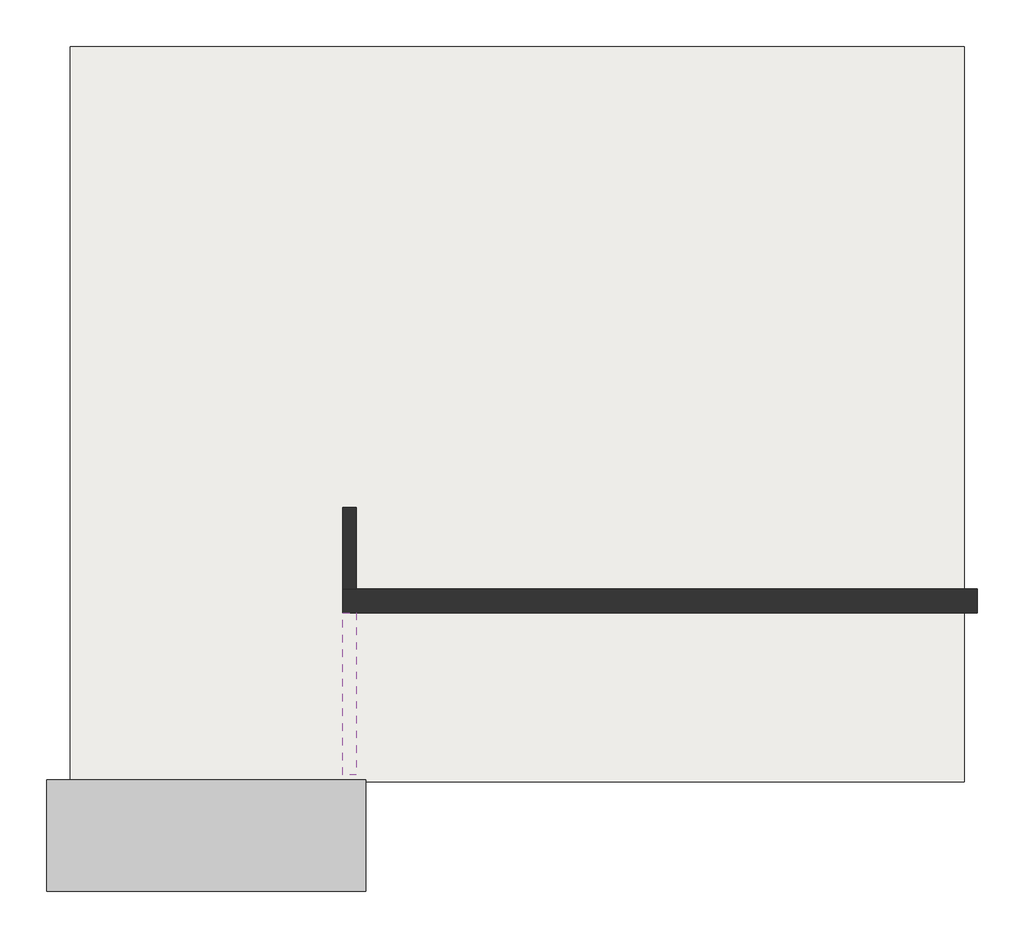
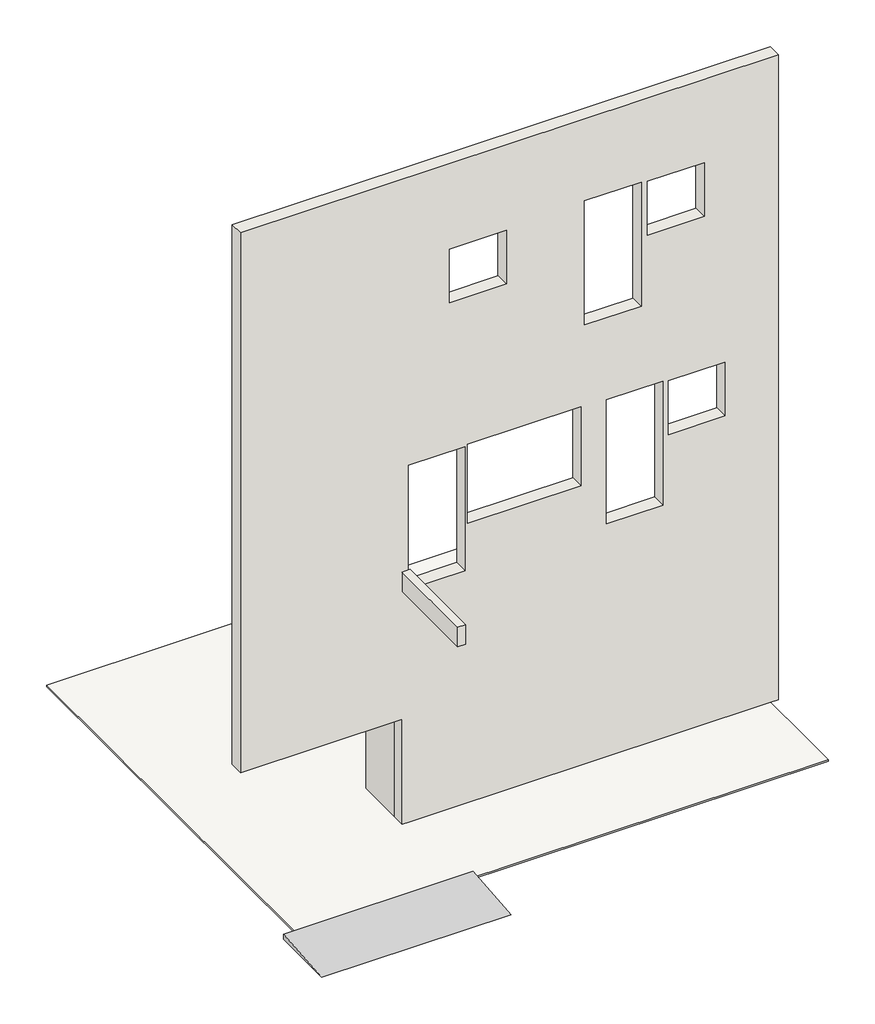
# One storey: 3 walls, 1 ramp, 1 slab.
"""IFC4 building model written with IfcOpenShell, lengths in millimetres."""

from ifc_helpers import new_model, si_unit, frame, origin, place, context, project, spatial, polyline, outline, extrude, faceted_brep, transform, mapped, element, save
from components import standard_ef43e6ca

model = new_model("IFC4")

# Units and contexts
model_context = context("Model", 3, world=origin())
ifc_project = project(units=[si_unit("LENGTHUNIT", "METRE", prefix="MILLI")], contexts=[model_context])

# Site, building, storey
site = spatial("IfcSite", under=ifc_project)
building = spatial("IfcBuilding", under=site)
storey = spatial("IfcBuildingStorey", under=building, Elevation=914.4)

# Ramp
placement = place(None, origin())
standard_shape = standard_ef43e6ca(model_context)
element("IfcRamp", 1, ObjectType="Standard", at=placement, inside=storey, context=model_context, shape_type="MappedRepresentation", body=[
    mapped(standard_shape, transform((0.0, 0.0, 0.0), x_axis=(1.0, 0.0, 0.0), y_axis=(0.0, 1.0, 0.0), z_axis=(0.0, 0.0, 1.0))),
])

# Slab
element("IfcSlab", 2, ObjectType="2\"", at=placement, inside=storey, context=model_context, shape_type="SweptSolid", body=[
    extrude(outline(polyline([(9321.1305046, -1515.8053244), (9321.1305046, -8538.9053244), (788.1495839, -8538.9053244), (788.1495839, -1515.8053244), (9321.1305046, -1515.8053244)])), frame((0.0, 0.0, 889.0), z_axis=(0.0, 0.0, 1.0), x_axis=(1.0, 0.0, 0.0)), (0.0, 0.0, 1.0), 25.4),
])

# Walls
element("IfcWall", 3, ObjectType="5\"", at=placement, inside=storey, context=model_context, shape_type="SweptSolid", body=[
    extrude(outline(polyline([(3517.0722446, -6926.0053244), (3517.0722446, -8475.4053244), (3390.0722446, -8475.4053244), (3390.0722446, -6926.0053244), (3517.0722446, -6926.0053244)])), frame((0.0, 0.0, 4876.8), z_axis=(0.0, 0.0, 1.0), x_axis=(1.0, 0.0, 0.0)), (0.0, 0.0, 1.0), 330.2),
])
element("IfcWall", 4, ObjectType="5\"", at=placement, inside=storey, context=model_context, shape_type="Brep", body=[
    faceted_brep([(3517.0722446, -6697.4053244, 4648.2), (3517.0722446, -6697.4053244, 914.4), (3517.0722446, -5918.2703867, 914.4), (3517.0722446, -5918.2703867, 4648.2), (3390.0722446, -6697.4053244, 914.4), (3390.0722446, -6697.4053244, 2706.0311436), (3390.0722446, -6697.4053244, 4648.2), (3390.0722446, -5918.2703867, 4648.2), (3390.0722446, -5918.2703867, 914.4)], [[[0, 1, 2, 3]], [[4, 5, 6, 7, 8]], [[2, 1, 4, 8]], [[3, 2, 8, 7]], [[0, 3, 7, 6]], [[0, 6, 5, 4, 1]]]),
])
element("IfcWall", 5, ObjectType="9\"", at=placement, inside=storey, context=model_context, shape_type="Brep", body=[
    faceted_brep([(3390.0722446, -6926.0053244, 914.4), (3517.0722446, -6926.0053244, 914.4), (9321.1305046, -6926.0053244, 914.4), (9448.1305046, -6926.0053244, 914.4), (9448.1305046, -6926.0053244, 4648.2), (9448.1305046, -6926.0053244, 11658.6), (9448.1305046, -6926.0053244, 11887.2), (788.1495839, -6926.0053244, 11887.2), (788.1495839, -6926.0053244, 11658.6), (788.1495839, -6926.0053244, 2706.0311436), (3390.0722446, -6926.0053244, 2706.0311436), (6328.3305046, -6926.0053244, 8382.0), (6328.3305046, -6926.0053244, 10492.0), (7238.3305046, -6926.0053244, 10492.0), (7238.3305046, -6926.0053244, 8382.0), (7339.9305046, -6926.0053244, 9555.3436332), (7339.9305046, -6926.0053244, 10469.7436332), (8254.3305046, -6926.0053244, 10469.7436332), (8254.3305046, -6926.0053244, 9555.3436332), (4152.0722446, -6926.0053244, 9520.5168667), (4152.0722446, -6926.0053244, 10434.9168667), (5066.4722446, -6926.0053244, 10434.9168667), (5066.4722446, -6926.0053244, 9520.5168667), (6678.7935362, -6926.0053244, 4876.1169892), (6678.7935362, -6926.0053244, 6986.1169892), (7588.7935362, -6926.0053244, 6986.1169892), (7588.7935362, -6926.0053244, 4876.1169892), (8589.4971961, -6926.0053244, 6043.5616728), (7675.0971961, -6926.0053244, 6043.5616728), (7675.0971961, -6926.0053244, 6957.9616728), (8589.4971961, -6926.0053244, 6957.9616728), (3494.2808585, -6926.0053244, 4876.1169892), (3494.2808585, -6926.0053244, 6986.1169892), (4404.2808585, -6926.0053244, 6986.1169892), (4404.2808585, -6926.0053244, 4876.1169892), (4443.5935362, -6926.0053244, 5664.8881482), (4443.5935362, -6926.0053244, 7011.0881482), (6272.3935362, -6926.0053244, 7011.0881482), (6272.3935362, -6926.0053244, 5664.8881482), (9448.1305046, -6697.4053244, 914.4), (9219.5305046, -6697.4053244, 914.4), (3517.0722446, -6697.4053244, 914.4), (3390.0722446, -6697.4053244, 914.4), (3390.0722446, -6697.4053244, 2706.0311436), (788.1495839, -6697.4053244, 2706.0311436), (788.1495839, -6697.4053244, 11887.2), (9448.1305046, -6697.4053244, 11887.2), (9448.1305046, -6697.4053244, 11658.6), (6328.3305046, -6697.4053244, 10492.0), (6328.3305046, -6697.4053244, 8382.0), (7238.3305046, -6697.4053244, 8382.0), (7238.3305046, -6697.4053244, 10492.0), (7339.9305046, -6697.4053244, 10469.7436332), (7339.9305046, -6697.4053244, 9555.3436332), (8254.3305046, -6697.4053244, 9555.3436332), (8254.3305046, -6697.4053244, 10469.7436332), (4152.0722446, -6697.4053244, 10434.9168667), (4152.0722446, -6697.4053244, 9520.5168667), (5066.4722446, -6697.4053244, 9520.5168667), (5066.4722446, -6697.4053244, 10434.9168667), (6678.7935362, -6697.4053244, 6986.1169892), (6678.7935362, -6697.4053244, 4876.1169892), (7588.7935362, -6697.4053244, 4876.1169892), (7588.7935362, -6697.4053244, 6986.1169892), (7675.0971961, -6697.4053244, 6043.5616728), (8589.4971961, -6697.4053244, 6043.5616728), (8589.4971961, -6697.4053244, 6957.9616728), (7675.0971961, -6697.4053244, 6957.9616728), (3494.2808585, -6697.4053244, 4876.1169892), (4404.2808585, -6697.4053244, 4876.1169892), (4404.2808585, -6697.4053244, 6986.1169892), (3494.2808585, -6697.4053244, 6986.1169892), (4443.5935362, -6697.4053244, 7011.0881482), (4443.5935362, -6697.4053244, 5664.8881482), (6272.3935362, -6697.4053244, 5664.8881482), (6272.3935362, -6697.4053244, 7011.0881482), (788.1495839, -6811.7053244, 2706.0311436)], [[[0, 1, 2, 3, 4, 5, 6, 7, 8, 9, 10], [11, 12, 13, 14], [15, 16, 17, 18], [19, 20, 21, 22], [23, 24, 25, 26], [27, 28, 29, 30], [31, 32, 33, 34], [35, 36, 37, 38]], [[39, 40, 41, 42, 43, 44, 45, 46, 47], [48, 49, 50, 51], [52, 53, 54, 55], [56, 57, 58, 59], [60, 61, 62, 63], [64, 65, 66, 67], [68, 69, 70, 71], [72, 73, 74, 75]], [[12, 11, 49, 48]], [[13, 12, 48, 51]], [[14, 13, 51, 50]], [[11, 14, 50, 49]], [[53, 52, 16, 15]], [[54, 53, 15, 18]], [[55, 54, 18, 17]], [[52, 55, 17, 16]], [[57, 56, 20, 19]], [[58, 57, 19, 22]], [[59, 58, 22, 21]], [[56, 59, 21, 20]], [[24, 23, 61, 60]], [[25, 24, 60, 63]], [[26, 25, 63, 62]], [[23, 26, 62, 61]], [[67, 29, 28, 64]], [[27, 65, 64, 28]], [[65, 27, 30, 66]], [[66, 30, 29, 67]], [[32, 31, 68, 71]], [[33, 32, 71, 70]], [[34, 33, 70, 69]], [[31, 34, 69, 68]], [[72, 36, 35, 73]], [[73, 35, 38, 74]], [[74, 38, 37, 75]], [[36, 72, 75, 37]], [[9, 8, 7, 45, 44, 76]], [[6, 5, 4, 3, 39, 47, 46]], [[3, 2, 1, 0, 42, 41, 40, 39]], [[7, 6, 46, 45]], [[10, 9, 76, 44, 43]], [[0, 10, 43, 42]]]),
])

save(model, "model.ifc")

# Revit data of these elements
# Type "Standard"
#   built-in parameter 1008304 = 0.492126 (stored number, unit not read)
#   built-in parameter 1008303 = 39.3701 (stored number, unit not read)
#   built-in parameter 1008301 = 12 (stored number, unit not read)
#   built-in parameter 1008305 = 1
#   Function = 0
# Type "2\""
#   Keynote = "E60/130"
#   Function = 0
#   Layers, outside or top first: 0' - 1" "Concrete, Precast" (function 1)
# Type "5\""
#   Keynote = "F10"
#   Layers, outside or top first: 0' - 5" "Concrete" (function 1)
# Type "9\""
#   Keynote = "F10"
#   Layers, outside or top first: 0' - 9" "Concrete" (function 1)
# Element 1 (IfcRamp, "Standard")
#   built-in parameter 1007275 = "DN"
#   built-in parameter 1007272 = "UP"
#   Width = 10' - 0"
#   built-in parameter 1007276 = 1
#   built-in parameter 1007274 = 1
#   built-in parameter 1007273 = 1
#   built-in parameter 1007271 = 1
#   Phase Created = New Construction
# Element 2 (IfcSlab, "2\"")
#   Height Offset From Level = 0' - 0"
#   Phase Created = New Construction
#   Materials on its faces: "Concrete, Precast"
# Element 3 (IfcWall, "5\"")
#   built-in parameter 1001111 = 13' - 0"
#   Top Offset = 0' - 0"
#   Base Offset = 13' - 0"
#   Unconnected Height = 1' - 1"
#   wall height = 1' - 1"
#   Phase Created = New Construction
#   Base Constraint = DRIVE LEV
#   Materials on its faces: "Concrete"
# Element 4 (IfcWall, "5\"")
#   Top Offset = 0' - 0"
#   Base Offset = 0' - 0"
#   Unconnected Height = 12' - 3"
#   wall height = 12' - 3"
#   Phase Created = New Construction
#   Base Constraint = DRIVE LEV
#   Materials on its faces: "Concrete"
# Element 5 (IfcWall, "9\"")
#   Top Offset = 0' - 0"
#   Base Offset = 0' - 0"
#   wall height = 36' - 0"
#   Phase Created = New Construction
#   Base Constraint = DRIVE LEV
#   Top Constraint = ROOF LEV
#   Materials on its faces: "Concrete", "Gypsum Wall Board"
# Materials
#   "Concrete, Precast": class "Concrete", colour RGB 192 192 192, transparency 0, Description = "Precast concrete", Cost = 0
#   "Concrete": class "Concrete", colour RGB 120 120 120, transparency 0, Description = "Portland Cement Concrete", Cost = 0
#   "Gypsum Wall Board": class "Generic", colour RGB 249 249 249, transparency 0, Description = "Gypsum Wall Board", Cost = 0
